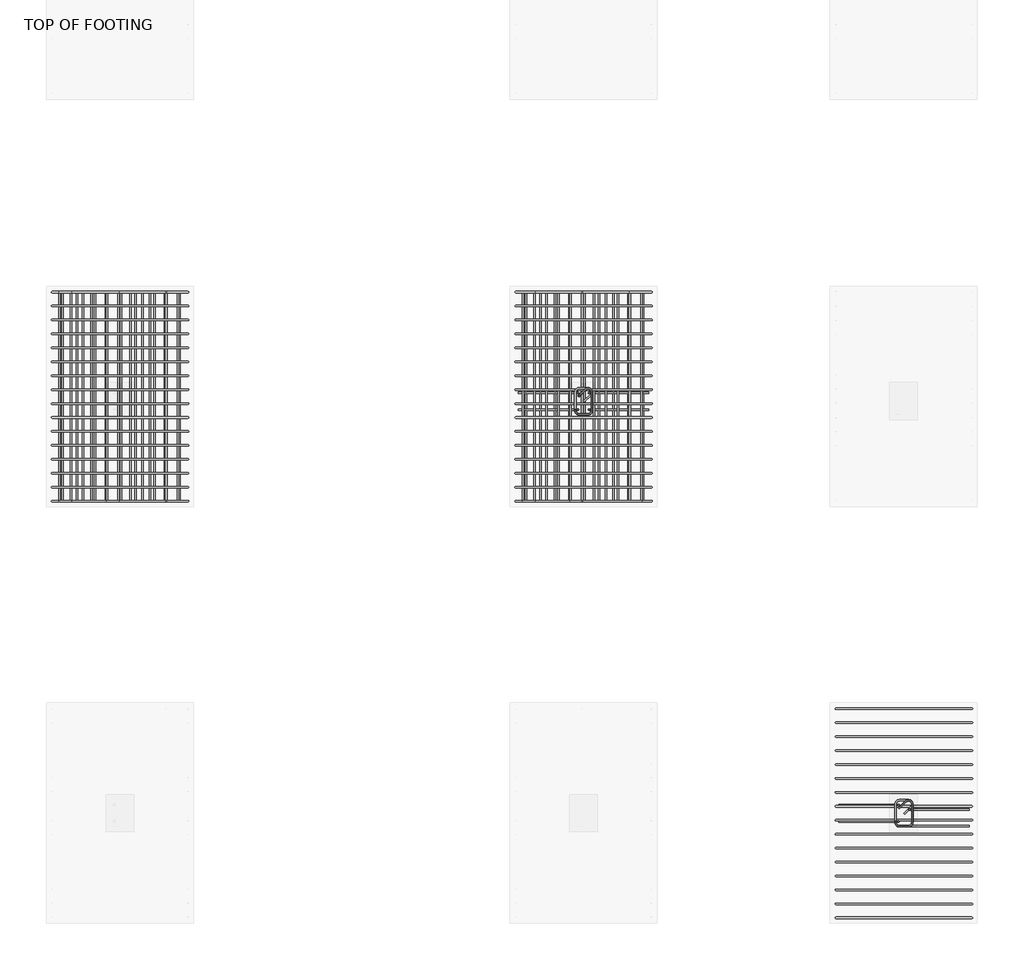
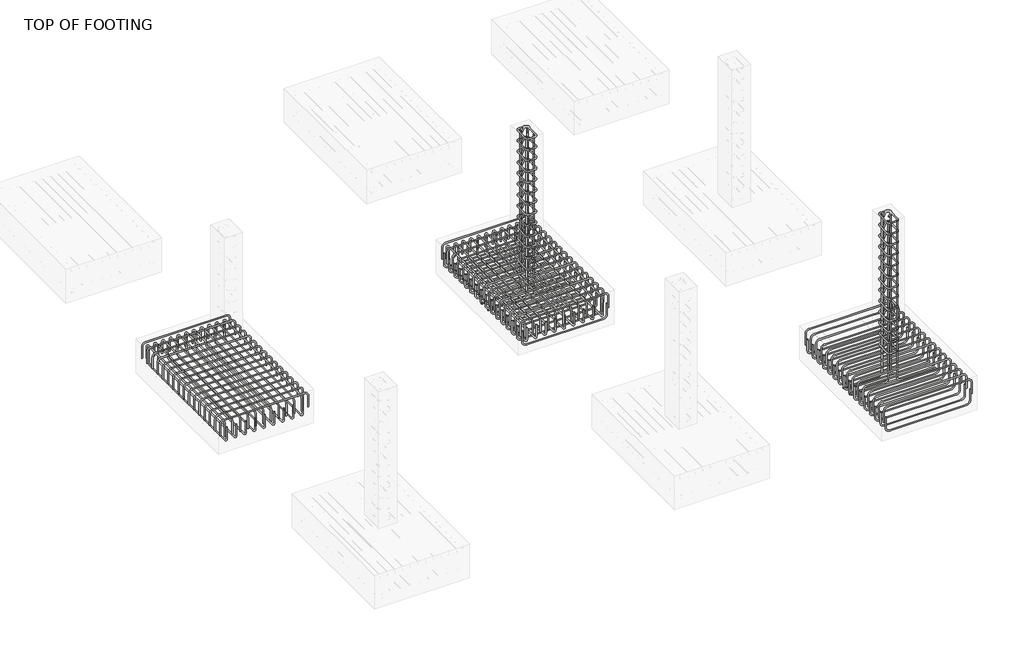
# One storey, part 6 of 8: 15 reinforcing bars.
"""IFC4 building model written with IfcOpenShell, lengths in millimetres."""

from ifc_helpers import new_model, si_unit, point, frame, origin, place, context, project, spatial, polyline, circle_curve, trimmed, segment, composite_curve, source, transform, mapped, element, save
from ifc_brep_helpers import swept_disk

model = new_model("IFC4")

# Units and contexts
model_context = context("Model", 3, world=origin())
ifc_project = project(units=[si_unit("LENGTHUNIT", "METRE", prefix="MILLI")], contexts=[model_context])

# Site, building, storey
site = spatial("IfcSite", under=ifc_project)
building = spatial("IfcBuilding", under=site)
storey = spatial("IfcBuildingStorey", under=building, Name="TOP OF FOOTING", Elevation=-1828.8)

# Reinforcing bars
placement = place(None, origin())
reinforcing_bar_shape = source(origin(), model_context, "Body", "SolidModel", [
    swept_disk(composite_curve([segment(polyline([(9462.2817577, 2235.4007933, -46.35), (9518.0253207, 2291.1443562, -46.35)]), True, "CONTINUOUS"), segment(trimmed(circle_curve(frame((9540.1931183, 2268.9765586, -46.35), z_axis=(0.0, 0.0, -1.0), x_axis=(-22.167797599999176, 22.167797600000085, 0.0)), 31.35), [point((9518.0253207, 2291.1443562, -46.35))], [point((9571.5431183, 2268.9765586, -46.35))], True, "CARTESIAN"), True, "CONTINUOUS"), segment(polyline([(9571.5431183, 2268.9765586, -46.35), (9571.5431183, 2119.5765586, -46.35)]), True, "CONTINUOUS"), segment(trimmed(circle_curve(frame((9540.1931183, 2119.5765586, -46.35), z_axis=(0.0, 0.0, -1.0), x_axis=(31.350000000000364, 0.0, 0.0)), 31.35), [point((9571.5431183, 2119.5765586, -46.35))], [point((9540.1931183, 2088.2265586, -46.35))], True, "CARTESIAN"), True, "CONTINUOUS"), segment(polyline([(9540.1931183, 2088.2265586, -46.35), (9466.9931183, 2088.2265586, -46.35)]), True, "CONTINUOUS"), segment(trimmed(circle_curve(frame((9466.9931183, 2119.5205096, -44.4761991), z_axis=(0.0, 0.05977036468717588, -0.9982121535551258), x_axis=(0.0, -31.293951000000106, -1.873800899999999)), 31.35), [point((9466.9931183, 2088.2265586, -46.35))], [point((9435.6431183, 2119.5205096, -44.4761991))], True, "CARTESIAN"), True, "CONTINUOUS"), segment(polyline([(9435.6431183, 2119.5205096, -44.4761991), (9435.6431183, 2269.0326076, -35.5238009)]), True, "CONTINUOUS"), segment(trimmed(circle_curve(frame((9466.9931183, 2269.0326076, -35.5238009), z_axis=(0.0, 0.05977036468717588, -0.9982121535551258), x_axis=(-31.350000000000364, 0.0, 0.0)), 31.35), [point((9435.6431183, 2269.0326076, -35.5238009))], [point((9466.9931183, 2300.3265586, -33.65))], True, "CARTESIAN"), True, "CONTINUOUS"), segment(polyline([(9466.9931183, 2300.3265586, -33.65), (9540.1931183, 2300.3265586, -33.65)]), True, "CONTINUOUS"), segment(trimmed(circle_curve(frame((9540.1931183, 2268.9765586, -33.65), z_axis=(0.0, 0.0, -1.0), x_axis=(0.0, 31.350000000000364, 0.0)), 31.35), [point((9540.1931183, 2300.3265586, -33.65))], [point((9562.3609159, 2246.808761, -33.65))], True, "CARTESIAN"), True, "CONTINUOUS"), segment(polyline([(9562.3609159, 2246.808761, -33.65), (9506.6173529, 2191.0651981, -33.65)]), True, "CONTINUOUS")], self_intersect=False), 6.35),
])
element("IfcReinforcingBar", 1, at=placement, inside=storey, context=model_context, shape_type="MappedRepresentation", body=[
    mapped(reinforcing_bar_shape, transform((0.0, 0.0, 0.0), x_axis=(1.0, 0.0, 0.0), y_axis=(0.0, 1.0, 0.0), z_axis=(0.0, 0.0, 1.0))),
    mapped(reinforcing_bar_shape, transform((0.0, 0.0, -144.675), x_axis=(1.0, 0.0, 0.0), y_axis=(0.0, 1.0, 0.0), z_axis=(0.0, 0.0, 1.0))),
    mapped(reinforcing_bar_shape, transform((0.0, 0.0, -289.35), x_axis=(1.0, 0.0, 0.0), y_axis=(0.0, 1.0, 0.0), z_axis=(0.0, 0.0, 1.0))),
    mapped(reinforcing_bar_shape, transform((0.0, 0.0, -434.025), x_axis=(1.0, 0.0, 0.0), y_axis=(0.0, 1.0, 0.0), z_axis=(0.0, 0.0, 1.0))),
    mapped(reinforcing_bar_shape, transform((0.0, 0.0, -578.7), x_axis=(1.0, 0.0, 0.0), y_axis=(0.0, 1.0, 0.0), z_axis=(0.0, 0.0, 1.0))),
    mapped(reinforcing_bar_shape, transform((0.0, 0.0, -723.375), x_axis=(1.0, 0.0, 0.0), y_axis=(0.0, 1.0, 0.0), z_axis=(0.0, 0.0, 1.0))),
    mapped(reinforcing_bar_shape, transform((0.0, 0.0, -868.05), x_axis=(1.0, 0.0, 0.0), y_axis=(0.0, 1.0, 0.0), z_axis=(0.0, 0.0, 1.0))),
    mapped(reinforcing_bar_shape, transform((0.0, 0.0, -1012.725), x_axis=(1.0, 0.0, 0.0), y_axis=(0.0, 1.0, 0.0), z_axis=(0.0, 0.0, 1.0))),
    mapped(reinforcing_bar_shape, transform((0.0, 0.0, -1157.4), x_axis=(1.0, 0.0, 0.0), y_axis=(0.0, 1.0, 0.0), z_axis=(0.0, 0.0, 1.0))),
    mapped(reinforcing_bar_shape, transform((0.0, 0.0, -1302.075), x_axis=(1.0, 0.0, 0.0), y_axis=(0.0, 1.0, 0.0), z_axis=(0.0, 0.0, 1.0))),
    mapped(reinforcing_bar_shape, transform((0.0, 0.0, -1446.75), x_axis=(1.0, 0.0, 0.0), y_axis=(0.0, 1.0, 0.0), z_axis=(0.0, 0.0, 1.0))),
    mapped(reinforcing_bar_shape, transform((0.0, 0.0, -1591.425), x_axis=(1.0, 0.0, 0.0), y_axis=(0.0, 1.0, 0.0), z_axis=(0.0, 0.0, 1.0))),
    mapped(reinforcing_bar_shape, transform((0.0, 0.0, -1736.1), x_axis=(1.0, 0.0, 0.0), y_axis=(0.0, 1.0, 0.0), z_axis=(0.0, 0.0, 1.0))),
])
reinforcing_bar_2_shape = source(origin(), model_context, "Body", "SolidModel", [
    swept_disk(composite_curve([segment(polyline([(10036.619602, 2088.2265586, -2177.1384798), (9595.4627797, 2088.2265586, -2177.1384798)]), True, "CONTINUOUS"), segment(trimmed(circle_curve(frame((9595.4627797, 2088.2265586, -2130.7884798), z_axis=(0.0, 1.0, 0.0), x_axis=(0.0, 0.0, -46.34999999999991)), 46.35), [point((9595.4627797, 2088.2265586, -2177.1384798))], [point((9549.1127797, 2088.2265586, -2130.7884798))], True, "CARTESIAN"), True, "CONTINUOUS"), segment(polyline([(9549.1127797, 2088.2265586, -2130.7884798), (9549.1127797, 2088.2265586, -40.0)]), True, "CONTINUOUS")], self_intersect=False), 6.35),
])
element("IfcReinforcingBar", 2, at=placement, inside=storey, context=model_context, shape_type="MappedRepresentation", body=[
    mapped(reinforcing_bar_2_shape, transform((0.0, 0.0, 0.0), x_axis=(1.0, 0.0, 0.0), y_axis=(0.0, 1.0, 0.0), z_axis=(0.0, 0.0, 1.0))),
    mapped(reinforcing_bar_2_shape, transform((0.0, 135.9, 0.0), x_axis=(1.0, 0.0, 0.0), y_axis=(0.0, 1.0, 0.0), z_axis=(0.0, 0.0, 1.0))),
])
reinforcing_bar_3_shape = source(origin(), model_context, "Body", "SolidModel", [
    swept_disk(composite_curve([segment(polyline([(8970.5666346, 2126.3265586, -2177.1384798), (9411.7234568, 2126.3265586, -2177.1384798)]), True, "CONTINUOUS"), segment(trimmed(circle_curve(frame((9411.7234568, 2126.3265586, -2130.7884798), z_axis=(0.0, -1.0, 0.0), x_axis=(0.0, 0.0, -46.34999999999991)), 46.35), [point((9411.7234568, 2126.3265586, -2177.1384798))], [point((9458.0734568, 2126.3265586, -2130.7884798))], True, "CARTESIAN"), True, "CONTINUOUS"), segment(polyline([(9458.0734568, 2126.3265586, -2130.7884798), (9458.0734568, 2126.3265586, -40.0)]), True, "CONTINUOUS")], self_intersect=False), 6.35),
])
element("IfcReinforcingBar", 3, at=placement, inside=storey, context=model_context, shape_type="MappedRepresentation", body=[
    mapped(reinforcing_bar_3_shape, transform((0.0, 0.0, 0.0), x_axis=(1.0, 0.0, 0.0), y_axis=(0.0, 1.0, 0.0), z_axis=(0.0, 0.0, 1.0))),
    mapped(reinforcing_bar_3_shape, transform((0.0, 135.9, 0.0), x_axis=(1.0, 0.0, 0.0), y_axis=(0.0, 1.0, 0.0), z_axis=(0.0, 0.0, 1.0))),
])
reinforcing_bar_4_shape = source(origin(), model_context, "Body", "SolidModel", [
    swept_disk(composite_curve([segment(polyline([(6846.0817577, 5600.7423139, -46.35), (6901.8253207, 5656.4858768, -46.35)]), True, "CONTINUOUS"), segment(trimmed(circle_curve(frame((6923.9931183, 5634.3180792, -46.35), z_axis=(0.0, 0.0, -1.0), x_axis=(-22.167797600000085, 22.167797600000085, 0.0)), 31.35), [point((6901.8253207, 5656.4858768, -46.35))], [point((6955.3431183, 5634.3180792, -46.35))], True, "CARTESIAN"), True, "CONTINUOUS"), segment(polyline([(6955.3431183, 5634.3180792, -46.35), (6955.3431183, 5484.9180792, -46.35)]), True, "CONTINUOUS"), segment(trimmed(circle_curve(frame((6923.9931183, 5484.9180792, -46.35), z_axis=(0.0, 0.0, -1.0), x_axis=(31.350000000000364, 0.0, 0.0)), 31.35), [point((6955.3431183, 5484.9180792, -46.35))], [point((6923.9931183, 5453.5680792, -46.35))], True, "CARTESIAN"), True, "CONTINUOUS"), segment(polyline([(6923.9931183, 5453.5680792, -46.35), (6850.7931183, 5453.5680792, -46.35)]), True, "CONTINUOUS"), segment(trimmed(circle_curve(frame((6850.7931183, 5484.8620303, -44.4761991), z_axis=(0.0, 0.05977036468717588, -0.9982121535551258), x_axis=(0.0, -31.293951099999504, -1.873800899999999)), 31.35), [point((6850.7931183, 5453.5680792, -46.35))], [point((6819.4431183, 5484.8620303, -44.4761991))], True, "CARTESIAN"), True, "CONTINUOUS"), segment(polyline([(6819.4431183, 5484.8620303, -44.4761991), (6819.4431183, 5634.3741282, -35.5238009)]), True, "CONTINUOUS"), segment(trimmed(circle_curve(frame((6850.7931183, 5634.3741282, -35.5238009), z_axis=(0.0, 0.05977036468717588, -0.9982121535551258), x_axis=(-31.350000000000364, 0.0, 0.0)), 31.35), [point((6819.4431183, 5634.3741282, -35.5238009))], [point((6850.7931183, 5665.6680792, -33.65))], True, "CARTESIAN"), True, "CONTINUOUS"), segment(polyline([(6850.7931183, 5665.6680792, -33.65), (6923.9931183, 5665.6680792, -33.65)]), True, "CONTINUOUS"), segment(trimmed(circle_curve(frame((6923.9931183, 5634.3180792, -33.65), z_axis=(0.0, 0.0, -1.0), x_axis=(0.0, 31.349999999999454, 0.0)), 31.35), [point((6923.9931183, 5665.6680792, -33.65))], [point((6946.1609159, 5612.1502816, -33.65))], True, "CARTESIAN"), True, "CONTINUOUS"), segment(polyline([(6946.1609159, 5612.1502816, -33.65), (6890.4173529, 5556.4067187, -33.65)]), True, "CONTINUOUS")], self_intersect=False), 6.35),
])
element("IfcReinforcingBar", 4, at=placement, inside=storey, context=model_context, shape_type="MappedRepresentation", body=[
    mapped(reinforcing_bar_4_shape, transform((0.0, 0.0, 0.0), x_axis=(1.0, 0.0, 0.0), y_axis=(0.0, 1.0, 0.0), z_axis=(0.0, 0.0, 1.0))),
    mapped(reinforcing_bar_4_shape, transform((0.0, 0.0, -144.675), x_axis=(1.0, 0.0, 0.0), y_axis=(0.0, 1.0, 0.0), z_axis=(0.0, 0.0, 1.0))),
    mapped(reinforcing_bar_4_shape, transform((0.0, 0.0, -289.35), x_axis=(1.0, 0.0, 0.0), y_axis=(0.0, 1.0, 0.0), z_axis=(0.0, 0.0, 1.0))),
    mapped(reinforcing_bar_4_shape, transform((0.0, 0.0, -434.025), x_axis=(1.0, 0.0, 0.0), y_axis=(0.0, 1.0, 0.0), z_axis=(0.0, 0.0, 1.0))),
    mapped(reinforcing_bar_4_shape, transform((0.0, 0.0, -578.7), x_axis=(1.0, 0.0, 0.0), y_axis=(0.0, 1.0, 0.0), z_axis=(0.0, 0.0, 1.0))),
    mapped(reinforcing_bar_4_shape, transform((0.0, 0.0, -723.375), x_axis=(1.0, 0.0, 0.0), y_axis=(0.0, 1.0, 0.0), z_axis=(0.0, 0.0, 1.0))),
    mapped(reinforcing_bar_4_shape, transform((0.0, 0.0, -868.05), x_axis=(1.0, 0.0, 0.0), y_axis=(0.0, 1.0, 0.0), z_axis=(0.0, 0.0, 1.0))),
    mapped(reinforcing_bar_4_shape, transform((0.0, 0.0, -1012.725), x_axis=(1.0, 0.0, 0.0), y_axis=(0.0, 1.0, 0.0), z_axis=(0.0, 0.0, 1.0))),
    mapped(reinforcing_bar_4_shape, transform((0.0, 0.0, -1157.4), x_axis=(1.0, 0.0, 0.0), y_axis=(0.0, 1.0, 0.0), z_axis=(0.0, 0.0, 1.0))),
    mapped(reinforcing_bar_4_shape, transform((0.0, 0.0, -1302.075), x_axis=(1.0, 0.0, 0.0), y_axis=(0.0, 1.0, 0.0), z_axis=(0.0, 0.0, 1.0))),
    mapped(reinforcing_bar_4_shape, transform((0.0, 0.0, -1446.75), x_axis=(1.0, 0.0, 0.0), y_axis=(0.0, 1.0, 0.0), z_axis=(0.0, 0.0, 1.0))),
    mapped(reinforcing_bar_4_shape, transform((0.0, 0.0, -1591.425), x_axis=(1.0, 0.0, 0.0), y_axis=(0.0, 1.0, 0.0), z_axis=(0.0, 0.0, 1.0))),
    mapped(reinforcing_bar_4_shape, transform((0.0, 0.0, -1736.1), x_axis=(1.0, 0.0, 0.0), y_axis=(0.0, 1.0, 0.0), z_axis=(0.0, 0.0, 1.0))),
])
reinforcing_bar_5_shape = source(origin(), model_context, "Body", "SolidModel", [
    swept_disk(composite_curve([segment(polyline([(7420.419602, 5491.6680792, -2177.1384798), (6979.2627797, 5491.6680792, -2177.1384798)]), True, "CONTINUOUS"), segment(trimmed(circle_curve(frame((6979.2627797, 5491.6680792, -2130.7884798), z_axis=(0.0, 1.0, 0.0), x_axis=(0.0, 0.0, -46.34999999999991)), 46.35), [point((6979.2627797, 5491.6680792, -2177.1384798))], [point((6932.9127797, 5491.6680792, -2130.7884798))], True, "CARTESIAN"), True, "CONTINUOUS"), segment(polyline([(6932.9127797, 5491.6680792, -2130.7884798), (6932.9127797, 5491.6680792, -40.0)]), True, "CONTINUOUS")], self_intersect=False), 6.35),
])
element("IfcReinforcingBar", 5, at=placement, inside=storey, context=model_context, shape_type="MappedRepresentation", body=[
    mapped(reinforcing_bar_5_shape, transform((0.0, 0.0, 0.0), x_axis=(1.0, 0.0, 0.0), y_axis=(0.0, 1.0, 0.0), z_axis=(0.0, 0.0, 1.0))),
    mapped(reinforcing_bar_5_shape, transform((0.0, 135.9, 0.0), x_axis=(1.0, 0.0, 0.0), y_axis=(0.0, 1.0, 0.0), z_axis=(0.0, 0.0, 1.0))),
])
reinforcing_bar_6_shape = source(origin(), model_context, "Body", "SolidModel", [
    swept_disk(composite_curve([segment(polyline([(6354.3666346, 5491.6680792, -2177.1384798), (6795.5234568, 5491.6680792, -2177.1384798)]), True, "CONTINUOUS"), segment(trimmed(circle_curve(frame((6795.5234568, 5491.6680792, -2130.7884798), z_axis=(0.0, -1.0, 0.0), x_axis=(0.0, 0.0, -46.34999999999991)), 46.35), [point((6795.5234568, 5491.6680792, -2177.1384798))], [point((6841.8734568, 5491.6680792, -2130.7884798))], True, "CARTESIAN"), True, "CONTINUOUS"), segment(polyline([(6841.8734568, 5491.6680792, -2130.7884798), (6841.8734568, 5491.6680792, -40.0)]), True, "CONTINUOUS")], self_intersect=False), 6.35),
])
element("IfcReinforcingBar", 6, at=placement, inside=storey, context=model_context, shape_type="MappedRepresentation", body=[
    mapped(reinforcing_bar_6_shape, transform((0.0, 0.0, 0.0), x_axis=(1.0, 0.0, 0.0), y_axis=(0.0, 1.0, 0.0), z_axis=(0.0, 0.0, 1.0))),
    mapped(reinforcing_bar_6_shape, transform((0.0, 135.9, 0.0), x_axis=(1.0, 0.0, 0.0), y_axis=(0.0, 1.0, 0.0), z_axis=(0.0, 0.0, 1.0))),
])
reinforcing_bar_7_shape = source(origin(), model_context, "Body", "SolidModel", [
    swept_disk(composite_curve([segment(polyline([(2549.1431183, 6451.7662126, -2068.8), (2549.1431183, 6451.7662126, -1921.5)]), True, "CONTINUOUS"), segment(trimmed(circle_curve(frame((2595.4931183, 6451.7662126, -1921.5), z_axis=(0.0, 1.0, 0.0), x_axis=(-46.34999999999991, 0.0, 0.0)), 46.35), [point((2549.1431183, 6451.7662126, -1921.5))], [point((2595.4931183, 6451.7662126, -1875.15))], True, "CARTESIAN"), True, "CONTINUOUS"), segment(polyline([(2595.4931183, 6451.7662126, -1875.15), (3610.0931183, 6451.7662126, -1875.15)]), True, "CONTINUOUS"), segment(trimmed(circle_curve(frame((3610.0931183, 6451.7662126, -1921.5), z_axis=(0.0, 1.0, 0.0), x_axis=(0.0, 0.0, 46.34999999999991)), 46.35), [point((3610.0931183, 6451.7662126, -1875.15))], [point((3656.4431183, 6451.7662126, -1921.5))], True, "CARTESIAN"), True, "CONTINUOUS"), segment(polyline([(3656.4431183, 6451.7662126, -1921.5), (3656.4431183, 6451.7662126, -2068.8)]), True, "CONTINUOUS")], self_intersect=False), 6.35),
])
element("IfcReinforcingBar", 7, at=placement, inside=storey, context=model_context, shape_type="MappedRepresentation", body=[
    mapped(reinforcing_bar_7_shape, transform((0.0, 0.0, 0.0), x_axis=(1.0, 0.0, 0.0), y_axis=(0.0, 1.0, 0.0), z_axis=(0.0, 0.0, 1.0))),
    mapped(reinforcing_bar_7_shape, transform((0.0, -113.82, 0.0), x_axis=(1.0, 0.0, 0.0), y_axis=(0.0, 1.0, 0.0), z_axis=(0.0, 0.0, 1.0))),
    mapped(reinforcing_bar_7_shape, transform((0.0, -227.64, 0.0), x_axis=(1.0, 0.0, 0.0), y_axis=(0.0, 1.0, 0.0), z_axis=(0.0, 0.0, 1.0))),
    mapped(reinforcing_bar_7_shape, transform((0.0, -341.46, 0.0), x_axis=(1.0, 0.0, 0.0), y_axis=(0.0, 1.0, 0.0), z_axis=(0.0, 0.0, 1.0))),
    mapped(reinforcing_bar_7_shape, transform((0.0, -455.28, 0.0), x_axis=(1.0, 0.0, 0.0), y_axis=(0.0, 1.0, 0.0), z_axis=(0.0, 0.0, 1.0))),
    mapped(reinforcing_bar_7_shape, transform((0.0, -569.1, 0.0), x_axis=(1.0, 0.0, 0.0), y_axis=(0.0, 1.0, 0.0), z_axis=(0.0, 0.0, 1.0))),
    mapped(reinforcing_bar_7_shape, transform((0.0, -682.92, 0.0), x_axis=(1.0, 0.0, 0.0), y_axis=(0.0, 1.0, 0.0), z_axis=(0.0, 0.0, 1.0))),
    mapped(reinforcing_bar_7_shape, transform((0.0, -796.74, 0.0), x_axis=(1.0, 0.0, 0.0), y_axis=(0.0, 1.0, 0.0), z_axis=(0.0, 0.0, 1.0))),
    mapped(reinforcing_bar_7_shape, transform((0.0, -910.56, 0.0), x_axis=(1.0, 0.0, 0.0), y_axis=(0.0, 1.0, 0.0), z_axis=(0.0, 0.0, 1.0))),
    mapped(reinforcing_bar_7_shape, transform((0.0, -1024.38, 0.0), x_axis=(1.0, 0.0, 0.0), y_axis=(0.0, 1.0, 0.0), z_axis=(0.0, 0.0, 1.0))),
    mapped(reinforcing_bar_7_shape, transform((0.0, -1138.2, 0.0), x_axis=(1.0, 0.0, 0.0), y_axis=(0.0, 1.0, 0.0), z_axis=(0.0, 0.0, 1.0))),
    mapped(reinforcing_bar_7_shape, transform((0.0, -1252.02, 0.0), x_axis=(1.0, 0.0, 0.0), y_axis=(0.0, 1.0, 0.0), z_axis=(0.0, 0.0, 1.0))),
    mapped(reinforcing_bar_7_shape, transform((0.0, -1365.84, 0.0), x_axis=(1.0, 0.0, 0.0), y_axis=(0.0, 1.0, 0.0), z_axis=(0.0, 0.0, 1.0))),
    mapped(reinforcing_bar_7_shape, transform((0.0, -1479.66, 0.0), x_axis=(1.0, 0.0, 0.0), y_axis=(0.0, 1.0, 0.0), z_axis=(0.0, 0.0, 1.0))),
    mapped(reinforcing_bar_7_shape, transform((0.0, -1593.48, 0.0), x_axis=(1.0, 0.0, 0.0), y_axis=(0.0, 1.0, 0.0), z_axis=(0.0, 0.0, 1.0))),
    mapped(reinforcing_bar_7_shape, transform((0.0, -1707.3, 0.0), x_axis=(1.0, 0.0, 0.0), y_axis=(0.0, 1.0, 0.0), z_axis=(0.0, 0.0, 1.0))),
])
reinforcing_bar_8_shape = source(origin(), model_context, "Body", "SolidModel", [
    swept_disk(composite_curve([segment(polyline([(2631.3651697, 6451.7662126, -1986.9111268), (2631.3651697, 6451.7662126, -2134.2111268)]), True, "CONTINUOUS"), segment(trimmed(circle_curve(frame((2631.3651697, 6405.4162126, -2134.2111268), z_axis=(-1.0, 0.0, 0.0), x_axis=(0.0, 46.349999999999454, 0.0)), 46.35), [point((2631.3651697, 6451.7662126, -2134.2111268))], [point((2631.3651697, 6405.4162126, -2180.5611268))], True, "CARTESIAN"), True, "CONTINUOUS"), segment(polyline([(2631.3651697, 6405.4162126, -2180.5611268), (2631.3651697, 4790.8162126, -2180.5611268)]), True, "CONTINUOUS"), segment(trimmed(circle_curve(frame((2631.3651697, 4790.8162126, -2134.2111268), z_axis=(-1.0, 0.0, 0.0), x_axis=(0.0, 0.0, -46.34999999999991)), 46.35), [point((2631.3651697, 4790.8162126, -2180.5611268))], [point((2631.3651697, 4744.4662126, -2134.2111268))], True, "CARTESIAN"), True, "CONTINUOUS"), segment(polyline([(2631.3651697, 4744.4662126, -2134.2111268), (2631.3651697, 4744.4662126, -1986.9111268)]), True, "CONTINUOUS")], self_intersect=False), 6.35),
])
element("IfcReinforcingBar", 8, at=placement, inside=storey, context=model_context, shape_type="MappedRepresentation", body=[
    mapped(reinforcing_bar_8_shape, transform((0.0, 0.0, 0.0), x_axis=(1.0, 0.0, 0.0), y_axis=(0.0, 1.0, 0.0), z_axis=(0.0, 0.0, 1.0))),
    mapped(reinforcing_bar_8_shape, transform((119.5564677, 0.0, 0.0), x_axis=(1.0, 0.0, 0.0), y_axis=(0.0, 1.0, 0.0), z_axis=(0.0, 0.0, 1.0))),
    mapped(reinforcing_bar_8_shape, transform((239.1129355, 0.0, 0.0), x_axis=(1.0, 0.0, 0.0), y_axis=(0.0, 1.0, 0.0), z_axis=(0.0, 0.0, 1.0))),
    mapped(reinforcing_bar_8_shape, transform((358.6694032, 0.0, 0.0), x_axis=(1.0, 0.0, 0.0), y_axis=(0.0, 1.0, 0.0), z_axis=(0.0, 0.0, 1.0))),
    mapped(reinforcing_bar_8_shape, transform((478.2258709, 0.0, 0.0), x_axis=(1.0, 0.0, 0.0), y_axis=(0.0, 1.0, 0.0), z_axis=(0.0, 0.0, 1.0))),
    mapped(reinforcing_bar_8_shape, transform((597.7823387, 0.0, 0.0), x_axis=(1.0, 0.0, 0.0), y_axis=(0.0, 1.0, 0.0), z_axis=(0.0, 0.0, 1.0))),
    mapped(reinforcing_bar_8_shape, transform((717.3388064, 0.0, 0.0), x_axis=(1.0, 0.0, 0.0), y_axis=(0.0, 1.0, 0.0), z_axis=(0.0, 0.0, 1.0))),
    mapped(reinforcing_bar_8_shape, transform((836.8952741, 0.0, 0.0), x_axis=(1.0, 0.0, 0.0), y_axis=(0.0, 1.0, 0.0), z_axis=(0.0, 0.0, 1.0))),
    mapped(reinforcing_bar_8_shape, transform((956.4517419, 0.0, 0.0), x_axis=(1.0, 0.0, 0.0), y_axis=(0.0, 1.0, 0.0), z_axis=(0.0, 0.0, 1.0))),
])
reinforcing_bar_9_shape = source(origin(), model_context, "Body", "SolidModel", [
    swept_disk(composite_curve([segment(polyline([(3577.1331701, 6451.7662126, -2094.8977257), (3577.1331701, 6451.7662126, -1947.5977257)]), True, "CONTINUOUS"), segment(trimmed(circle_curve(frame((3577.1331701, 6405.4162126, -1947.5977257), z_axis=(1.0, 0.0, 0.0), x_axis=(0.0, 46.349999999999454, 0.0)), 46.35), [point((3577.1331701, 6451.7662126, -1947.5977257))], [point((3577.1331701, 6405.4162126, -1901.2477257))], True, "CARTESIAN"), True, "CONTINUOUS"), segment(polyline([(3577.1331701, 6405.4162126, -1901.2477257), (3577.1331701, 4790.8162126, -1901.2477257)]), True, "CONTINUOUS"), segment(trimmed(circle_curve(frame((3577.1331701, 4790.8162126, -1947.5977257), z_axis=(1.0, 0.0, 0.0), x_axis=(0.0, 0.0, 46.34999999999991)), 46.35), [point((3577.1331701, 4790.8162126, -1901.2477257))], [point((3577.1331701, 4744.4662126, -1947.5977257))], True, "CARTESIAN"), True, "CONTINUOUS"), segment(polyline([(3577.1331701, 4744.4662126, -1947.5977257), (3577.1331701, 4744.4662126, -2094.8977257)]), True, "CONTINUOUS")], self_intersect=False), 6.35),
])
element("IfcReinforcingBar", 9, at=placement, inside=storey, context=model_context, shape_type="MappedRepresentation", body=[
    mapped(reinforcing_bar_9_shape, transform((0.0, 0.0, 0.0), x_axis=(1.0, 0.0, 0.0), y_axis=(0.0, 1.0, 0.0), z_axis=(0.0, 0.0, 1.0))),
    mapped(reinforcing_bar_9_shape, transform((-97.0050815, 0.0, 0.0), x_axis=(1.0, 0.0, 0.0), y_axis=(0.0, 1.0, 0.0), z_axis=(0.0, 0.0, 1.0))),
    mapped(reinforcing_bar_9_shape, transform((-194.0101631, 0.0, 0.0), x_axis=(1.0, 0.0, 0.0), y_axis=(0.0, 1.0, 0.0), z_axis=(0.0, 0.0, 1.0))),
    mapped(reinforcing_bar_9_shape, transform((-291.0152446, 0.0, 0.0), x_axis=(1.0, 0.0, 0.0), y_axis=(0.0, 1.0, 0.0), z_axis=(0.0, 0.0, 1.0))),
    mapped(reinforcing_bar_9_shape, transform((-388.0203261, 0.0, 0.0), x_axis=(1.0, 0.0, 0.0), y_axis=(0.0, 1.0, 0.0), z_axis=(0.0, 0.0, 1.0))),
    mapped(reinforcing_bar_9_shape, transform((-485.0254076, 0.0, 0.0), x_axis=(1.0, 0.0, 0.0), y_axis=(0.0, 1.0, 0.0), z_axis=(0.0, 0.0, 1.0))),
    mapped(reinforcing_bar_9_shape, transform((-582.0304892, 0.0, 0.0), x_axis=(1.0, 0.0, 0.0), y_axis=(0.0, 1.0, 0.0), z_axis=(0.0, 0.0, 1.0))),
    mapped(reinforcing_bar_9_shape, transform((-679.0355707, 0.0, 0.0), x_axis=(1.0, 0.0, 0.0), y_axis=(0.0, 1.0, 0.0), z_axis=(0.0, 0.0, 1.0))),
    mapped(reinforcing_bar_9_shape, transform((-776.0406522, 0.0, 0.0), x_axis=(1.0, 0.0, 0.0), y_axis=(0.0, 1.0, 0.0), z_axis=(0.0, 0.0, 1.0))),
    mapped(reinforcing_bar_9_shape, transform((-873.0457338, 0.0, 0.0), x_axis=(1.0, 0.0, 0.0), y_axis=(0.0, 1.0, 0.0), z_axis=(0.0, 0.0, 1.0))),
    mapped(reinforcing_bar_9_shape, transform((-970.0508153, 0.0, 0.0), x_axis=(1.0, 0.0, 0.0), y_axis=(0.0, 1.0, 0.0), z_axis=(0.0, 0.0, 1.0))),
])
reinforcing_bar_10_shape = source(origin(), model_context, "Body", "SolidModel", [
    swept_disk(composite_curve([segment(polyline([(7421.6426771, 6451.7662126, -2008.2544267), (7421.6426771, 6451.7662126, -2155.5544267)]), True, "CONTINUOUS"), segment(trimmed(circle_curve(frame((7375.2926771, 6451.7662126, -2155.5544267), z_axis=(0.0, 1.0, 0.0), x_axis=(46.349999999999454, 0.0, 0.0)), 46.35), [point((7421.6426771, 6451.7662126, -2155.5544267))], [point((7375.2926771, 6451.7662126, -2201.9044267))], True, "CARTESIAN"), True, "CONTINUOUS"), segment(polyline([(7375.2926771, 6451.7662126, -2201.9044267), (6404.2766408, 6451.7662126, -2201.9044267)]), True, "CONTINUOUS"), segment(trimmed(circle_curve(frame((6404.2766408, 6451.7662126, -2155.5544267), z_axis=(0.0, 1.0, 0.0), x_axis=(0.0, 0.0, -46.34999999999991)), 46.35), [point((6404.2766408, 6451.7662126, -2201.9044267))], [point((6357.9266408, 6451.7662126, -2155.5544267))], True, "CARTESIAN"), True, "CONTINUOUS"), segment(polyline([(6357.9266408, 6451.7662126, -2155.5544267), (6357.9266408, 6451.7662126, -2008.2544267)]), True, "CONTINUOUS")], self_intersect=False), 6.35),
])
element("IfcReinforcingBar", 10, at=placement, inside=storey, context=model_context, shape_type="MappedRepresentation", body=[
    mapped(reinforcing_bar_10_shape, transform((0.0, 0.0, 0.0), x_axis=(1.0, 0.0, 0.0), y_axis=(0.0, 1.0, 0.0), z_axis=(0.0, 0.0, 1.0))),
    mapped(reinforcing_bar_10_shape, transform((0.0, -113.82, 0.0), x_axis=(1.0, 0.0, 0.0), y_axis=(0.0, 1.0, 0.0), z_axis=(0.0, 0.0, 1.0))),
    mapped(reinforcing_bar_10_shape, transform((0.0, -227.64, 0.0), x_axis=(1.0, 0.0, 0.0), y_axis=(0.0, 1.0, 0.0), z_axis=(0.0, 0.0, 1.0))),
    mapped(reinforcing_bar_10_shape, transform((0.0, -341.46, 0.0), x_axis=(1.0, 0.0, 0.0), y_axis=(0.0, 1.0, 0.0), z_axis=(0.0, 0.0, 1.0))),
    mapped(reinforcing_bar_10_shape, transform((0.0, -455.28, 0.0), x_axis=(1.0, 0.0, 0.0), y_axis=(0.0, 1.0, 0.0), z_axis=(0.0, 0.0, 1.0))),
    mapped(reinforcing_bar_10_shape, transform((0.0, -569.1, 0.0), x_axis=(1.0, 0.0, 0.0), y_axis=(0.0, 1.0, 0.0), z_axis=(0.0, 0.0, 1.0))),
    mapped(reinforcing_bar_10_shape, transform((0.0, -682.92, 0.0), x_axis=(1.0, 0.0, 0.0), y_axis=(0.0, 1.0, 0.0), z_axis=(0.0, 0.0, 1.0))),
    mapped(reinforcing_bar_10_shape, transform((0.0, -796.74, 0.0), x_axis=(1.0, 0.0, 0.0), y_axis=(0.0, 1.0, 0.0), z_axis=(0.0, 0.0, 1.0))),
    mapped(reinforcing_bar_10_shape, transform((0.0, -910.56, 0.0), x_axis=(1.0, 0.0, 0.0), y_axis=(0.0, 1.0, 0.0), z_axis=(0.0, 0.0, 1.0))),
    mapped(reinforcing_bar_10_shape, transform((0.0, -1024.38, 0.0), x_axis=(1.0, 0.0, 0.0), y_axis=(0.0, 1.0, 0.0), z_axis=(0.0, 0.0, 1.0))),
    mapped(reinforcing_bar_10_shape, transform((0.0, -1138.2, 0.0), x_axis=(1.0, 0.0, 0.0), y_axis=(0.0, 1.0, 0.0), z_axis=(0.0, 0.0, 1.0))),
    mapped(reinforcing_bar_10_shape, transform((0.0, -1252.02, 0.0), x_axis=(1.0, 0.0, 0.0), y_axis=(0.0, 1.0, 0.0), z_axis=(0.0, 0.0, 1.0))),
    mapped(reinforcing_bar_10_shape, transform((0.0, -1365.84, 0.0), x_axis=(1.0, 0.0, 0.0), y_axis=(0.0, 1.0, 0.0), z_axis=(0.0, 0.0, 1.0))),
    mapped(reinforcing_bar_10_shape, transform((0.0, -1479.66, 0.0), x_axis=(1.0, 0.0, 0.0), y_axis=(0.0, 1.0, 0.0), z_axis=(0.0, 0.0, 1.0))),
    mapped(reinforcing_bar_10_shape, transform((0.0, -1593.48, 0.0), x_axis=(1.0, 0.0, 0.0), y_axis=(0.0, 1.0, 0.0), z_axis=(0.0, 0.0, 1.0))),
    mapped(reinforcing_bar_10_shape, transform((0.0, -1707.3, 0.0), x_axis=(1.0, 0.0, 0.0), y_axis=(0.0, 1.0, 0.0), z_axis=(0.0, 0.0, 1.0))),
])
reinforcing_bar_11_shape = source(origin(), model_context, "Body", "SolidModel", [
    swept_disk(composite_curve([segment(polyline([(6333.7431183, 6451.7662126, -2068.8), (6333.7431183, 6451.7662126, -1921.5)]), True, "CONTINUOUS"), segment(trimmed(circle_curve(frame((6380.0931183, 6451.7662126, -1921.5), z_axis=(0.0, 1.0, 0.0), x_axis=(-46.350000000000364, 0.0, 0.0)), 46.35), [point((6333.7431183, 6451.7662126, -1921.5))], [point((6380.0931183, 6451.7662126, -1875.15))], True, "CARTESIAN"), True, "CONTINUOUS"), segment(polyline([(6380.0931183, 6451.7662126, -1875.15), (7394.6931183, 6451.7662126, -1875.15)]), True, "CONTINUOUS"), segment(trimmed(circle_curve(frame((7394.6931183, 6451.7662126, -1921.5), z_axis=(0.0, 1.0, 0.0), x_axis=(0.0, 0.0, 46.34999999999991)), 46.35), [point((7394.6931183, 6451.7662126, -1875.15))], [point((7441.0431183, 6451.7662126, -1921.5))], True, "CARTESIAN"), True, "CONTINUOUS"), segment(polyline([(7441.0431183, 6451.7662126, -1921.5), (7441.0431183, 6451.7662126, -2068.8)]), True, "CONTINUOUS")], self_intersect=False), 6.35),
])
element("IfcReinforcingBar", 11, at=placement, inside=storey, context=model_context, shape_type="MappedRepresentation", body=[
    mapped(reinforcing_bar_11_shape, transform((0.0, 0.0, 0.0), x_axis=(1.0, 0.0, 0.0), y_axis=(0.0, 1.0, 0.0), z_axis=(0.0, 0.0, 1.0))),
    mapped(reinforcing_bar_11_shape, transform((0.0, -113.82, 0.0), x_axis=(1.0, 0.0, 0.0), y_axis=(0.0, 1.0, 0.0), z_axis=(0.0, 0.0, 1.0))),
    mapped(reinforcing_bar_11_shape, transform((0.0, -227.64, 0.0), x_axis=(1.0, 0.0, 0.0), y_axis=(0.0, 1.0, 0.0), z_axis=(0.0, 0.0, 1.0))),
    mapped(reinforcing_bar_11_shape, transform((0.0, -341.46, 0.0), x_axis=(1.0, 0.0, 0.0), y_axis=(0.0, 1.0, 0.0), z_axis=(0.0, 0.0, 1.0))),
    mapped(reinforcing_bar_11_shape, transform((0.0, -455.28, 0.0), x_axis=(1.0, 0.0, 0.0), y_axis=(0.0, 1.0, 0.0), z_axis=(0.0, 0.0, 1.0))),
    mapped(reinforcing_bar_11_shape, transform((0.0, -569.1, 0.0), x_axis=(1.0, 0.0, 0.0), y_axis=(0.0, 1.0, 0.0), z_axis=(0.0, 0.0, 1.0))),
    mapped(reinforcing_bar_11_shape, transform((0.0, -682.92, 0.0), x_axis=(1.0, 0.0, 0.0), y_axis=(0.0, 1.0, 0.0), z_axis=(0.0, 0.0, 1.0))),
    mapped(reinforcing_bar_11_shape, transform((0.0, -796.74, 0.0), x_axis=(1.0, 0.0, 0.0), y_axis=(0.0, 1.0, 0.0), z_axis=(0.0, 0.0, 1.0))),
    mapped(reinforcing_bar_11_shape, transform((0.0, -910.56, 0.0), x_axis=(1.0, 0.0, 0.0), y_axis=(0.0, 1.0, 0.0), z_axis=(0.0, 0.0, 1.0))),
    mapped(reinforcing_bar_11_shape, transform((0.0, -1024.38, 0.0), x_axis=(1.0, 0.0, 0.0), y_axis=(0.0, 1.0, 0.0), z_axis=(0.0, 0.0, 1.0))),
    mapped(reinforcing_bar_11_shape, transform((0.0, -1138.2, 0.0), x_axis=(1.0, 0.0, 0.0), y_axis=(0.0, 1.0, 0.0), z_axis=(0.0, 0.0, 1.0))),
    mapped(reinforcing_bar_11_shape, transform((0.0, -1252.02, 0.0), x_axis=(1.0, 0.0, 0.0), y_axis=(0.0, 1.0, 0.0), z_axis=(0.0, 0.0, 1.0))),
    mapped(reinforcing_bar_11_shape, transform((0.0, -1365.84, 0.0), x_axis=(1.0, 0.0, 0.0), y_axis=(0.0, 1.0, 0.0), z_axis=(0.0, 0.0, 1.0))),
    mapped(reinforcing_bar_11_shape, transform((0.0, -1479.66, 0.0), x_axis=(1.0, 0.0, 0.0), y_axis=(0.0, 1.0, 0.0), z_axis=(0.0, 0.0, 1.0))),
    mapped(reinforcing_bar_11_shape, transform((0.0, -1593.48, 0.0), x_axis=(1.0, 0.0, 0.0), y_axis=(0.0, 1.0, 0.0), z_axis=(0.0, 0.0, 1.0))),
    mapped(reinforcing_bar_11_shape, transform((0.0, -1707.3, 0.0), x_axis=(1.0, 0.0, 0.0), y_axis=(0.0, 1.0, 0.0), z_axis=(0.0, 0.0, 1.0))),
])
reinforcing_bar_12_shape = source(origin(), model_context, "Body", "SolidModel", [
    swept_disk(composite_curve([segment(polyline([(6415.9651697, 6451.7662126, -1986.9111268), (6415.9651697, 6451.7662126, -2134.2111268)]), True, "CONTINUOUS"), segment(trimmed(circle_curve(frame((6415.9651697, 6405.4162126, -2134.2111268), z_axis=(-1.0, 0.0, 0.0), x_axis=(0.0, 46.349999999999454, 0.0)), 46.35), [point((6415.9651697, 6451.7662126, -2134.2111268))], [point((6415.9651697, 6405.4162126, -2180.5611268))], True, "CARTESIAN"), True, "CONTINUOUS"), segment(polyline([(6415.9651697, 6405.4162126, -2180.5611268), (6415.9651697, 4790.8162126, -2180.5611268)]), True, "CONTINUOUS"), segment(trimmed(circle_curve(frame((6415.9651697, 4790.8162126, -2134.2111268), z_axis=(-1.0, 0.0, 0.0), x_axis=(0.0, 0.0, -46.34999999999991)), 46.35), [point((6415.9651697, 4790.8162126, -2180.5611268))], [point((6415.9651697, 4744.4662126, -2134.2111268))], True, "CARTESIAN"), True, "CONTINUOUS"), segment(polyline([(6415.9651697, 4744.4662126, -2134.2111268), (6415.9651697, 4744.4662126, -1986.9111268)]), True, "CONTINUOUS")], self_intersect=False), 6.35),
])
element("IfcReinforcingBar", 12, at=placement, inside=storey, context=model_context, shape_type="MappedRepresentation", body=[
    mapped(reinforcing_bar_12_shape, transform((0.0, 0.0, 0.0), x_axis=(1.0, 0.0, 0.0), y_axis=(0.0, 1.0, 0.0), z_axis=(0.0, 0.0, 1.0))),
    mapped(reinforcing_bar_12_shape, transform((119.5564677, 0.0, 0.0), x_axis=(1.0, 0.0, 0.0), y_axis=(0.0, 1.0, 0.0), z_axis=(0.0, 0.0, 1.0))),
    mapped(reinforcing_bar_12_shape, transform((239.1129355, 0.0, 0.0), x_axis=(1.0, 0.0, 0.0), y_axis=(0.0, 1.0, 0.0), z_axis=(0.0, 0.0, 1.0))),
    mapped(reinforcing_bar_12_shape, transform((358.6694032, 0.0, 0.0), x_axis=(1.0, 0.0, 0.0), y_axis=(0.0, 1.0, 0.0), z_axis=(0.0, 0.0, 1.0))),
    mapped(reinforcing_bar_12_shape, transform((478.2258709, 0.0, 0.0), x_axis=(1.0, 0.0, 0.0), y_axis=(0.0, 1.0, 0.0), z_axis=(0.0, 0.0, 1.0))),
    mapped(reinforcing_bar_12_shape, transform((597.7823387, 0.0, 0.0), x_axis=(1.0, 0.0, 0.0), y_axis=(0.0, 1.0, 0.0), z_axis=(0.0, 0.0, 1.0))),
    mapped(reinforcing_bar_12_shape, transform((717.3388064, 0.0, 0.0), x_axis=(1.0, 0.0, 0.0), y_axis=(0.0, 1.0, 0.0), z_axis=(0.0, 0.0, 1.0))),
    mapped(reinforcing_bar_12_shape, transform((836.8952741, 0.0, 0.0), x_axis=(1.0, 0.0, 0.0), y_axis=(0.0, 1.0, 0.0), z_axis=(0.0, 0.0, 1.0))),
    mapped(reinforcing_bar_12_shape, transform((956.4517419, 0.0, 0.0), x_axis=(1.0, 0.0, 0.0), y_axis=(0.0, 1.0, 0.0), z_axis=(0.0, 0.0, 1.0))),
])
reinforcing_bar_13_shape = source(origin(), model_context, "Body", "SolidModel", [
    swept_disk(composite_curve([segment(polyline([(7361.7331701, 6451.7662126, -2094.8977257), (7361.7331701, 6451.7662126, -1947.5977257)]), True, "CONTINUOUS"), segment(trimmed(circle_curve(frame((7361.7331701, 6405.4162126, -1947.5977257), z_axis=(1.0, 0.0, 0.0), x_axis=(0.0, 46.349999999999454, 0.0)), 46.35), [point((7361.7331701, 6451.7662126, -1947.5977257))], [point((7361.7331701, 6405.4162126, -1901.2477257))], True, "CARTESIAN"), True, "CONTINUOUS"), segment(polyline([(7361.7331701, 6405.4162126, -1901.2477257), (7361.7331701, 4790.8162126, -1901.2477257)]), True, "CONTINUOUS"), segment(trimmed(circle_curve(frame((7361.7331701, 4790.8162126, -1947.5977257), z_axis=(1.0, 0.0, 0.0), x_axis=(0.0, 0.0, 46.34999999999991)), 46.35), [point((7361.7331701, 4790.8162126, -1901.2477257))], [point((7361.7331701, 4744.4662126, -1947.5977257))], True, "CARTESIAN"), True, "CONTINUOUS"), segment(polyline([(7361.7331701, 4744.4662126, -1947.5977257), (7361.7331701, 4744.4662126, -2094.8977257)]), True, "CONTINUOUS")], self_intersect=False), 6.35),
])
element("IfcReinforcingBar", 13, at=placement, inside=storey, context=model_context, shape_type="MappedRepresentation", body=[
    mapped(reinforcing_bar_13_shape, transform((0.0, 0.0, 0.0), x_axis=(1.0, 0.0, 0.0), y_axis=(0.0, 1.0, 0.0), z_axis=(0.0, 0.0, 1.0))),
    mapped(reinforcing_bar_13_shape, transform((-97.0050815, 0.0, 0.0), x_axis=(1.0, 0.0, 0.0), y_axis=(0.0, 1.0, 0.0), z_axis=(0.0, 0.0, 1.0))),
    mapped(reinforcing_bar_13_shape, transform((-194.0101631, 0.0, 0.0), x_axis=(1.0, 0.0, 0.0), y_axis=(0.0, 1.0, 0.0), z_axis=(0.0, 0.0, 1.0))),
    mapped(reinforcing_bar_13_shape, transform((-291.0152446, 0.0, 0.0), x_axis=(1.0, 0.0, 0.0), y_axis=(0.0, 1.0, 0.0), z_axis=(0.0, 0.0, 1.0))),
    mapped(reinforcing_bar_13_shape, transform((-388.0203261, 0.0, 0.0), x_axis=(1.0, 0.0, 0.0), y_axis=(0.0, 1.0, 0.0), z_axis=(0.0, 0.0, 1.0))),
    mapped(reinforcing_bar_13_shape, transform((-485.0254076, 0.0, 0.0), x_axis=(1.0, 0.0, 0.0), y_axis=(0.0, 1.0, 0.0), z_axis=(0.0, 0.0, 1.0))),
    mapped(reinforcing_bar_13_shape, transform((-582.0304892, 0.0, 0.0), x_axis=(1.0, 0.0, 0.0), y_axis=(0.0, 1.0, 0.0), z_axis=(0.0, 0.0, 1.0))),
    mapped(reinforcing_bar_13_shape, transform((-679.0355707, 0.0, 0.0), x_axis=(1.0, 0.0, 0.0), y_axis=(0.0, 1.0, 0.0), z_axis=(0.0, 0.0, 1.0))),
    mapped(reinforcing_bar_13_shape, transform((-776.0406522, 0.0, 0.0), x_axis=(1.0, 0.0, 0.0), y_axis=(0.0, 1.0, 0.0), z_axis=(0.0, 0.0, 1.0))),
    mapped(reinforcing_bar_13_shape, transform((-873.0457338, 0.0, 0.0), x_axis=(1.0, 0.0, 0.0), y_axis=(0.0, 1.0, 0.0), z_axis=(0.0, 0.0, 1.0))),
    mapped(reinforcing_bar_13_shape, transform((-970.0508153, 0.0, 0.0), x_axis=(1.0, 0.0, 0.0), y_axis=(0.0, 1.0, 0.0), z_axis=(0.0, 0.0, 1.0))),
])
reinforcing_bar_14_shape = source(origin(), model_context, "Body", "SolidModel", [
    swept_disk(composite_curve([segment(polyline([(10037.8426771, 3047.9265586, -2008.2544267), (10037.8426771, 3047.9265586, -2155.5544267)]), True, "CONTINUOUS"), segment(trimmed(circle_curve(frame((9991.4926771, 3047.9265586, -2155.5544267), z_axis=(0.0, 1.0, 0.0), x_axis=(46.350000000000364, 0.0, 0.0)), 46.35), [point((10037.8426771, 3047.9265586, -2155.5544267))], [point((9991.4926771, 3047.9265586, -2201.9044267))], True, "CARTESIAN"), True, "CONTINUOUS"), segment(polyline([(9991.4926771, 3047.9265586, -2201.9044267), (9020.4766408, 3047.9265586, -2201.9044267)]), True, "CONTINUOUS"), segment(trimmed(circle_curve(frame((9020.4766408, 3047.9265586, -2155.5544267), z_axis=(0.0, 1.0, 0.0), x_axis=(0.0, 0.0, -46.34999999999991)), 46.35), [point((9020.4766408, 3047.9265586, -2201.9044267))], [point((8974.1266408, 3047.9265586, -2155.5544267))], True, "CARTESIAN"), True, "CONTINUOUS"), segment(polyline([(8974.1266408, 3047.9265586, -2155.5544267), (8974.1266408, 3047.9265586, -2008.2544267)]), True, "CONTINUOUS")], self_intersect=False), 6.35),
])
element("IfcReinforcingBar", 14, at=placement, inside=storey, context=model_context, shape_type="MappedRepresentation", body=[
    mapped(reinforcing_bar_14_shape, transform((0.0, 0.0, 0.0), x_axis=(1.0, 0.0, 0.0), y_axis=(0.0, 1.0, 0.0), z_axis=(0.0, 0.0, 1.0))),
    mapped(reinforcing_bar_14_shape, transform((0.0, -113.82, 0.0), x_axis=(1.0, 0.0, 0.0), y_axis=(0.0, 1.0, 0.0), z_axis=(0.0, 0.0, 1.0))),
    mapped(reinforcing_bar_14_shape, transform((0.0, -227.64, 0.0), x_axis=(1.0, 0.0, 0.0), y_axis=(0.0, 1.0, 0.0), z_axis=(0.0, 0.0, 1.0))),
    mapped(reinforcing_bar_14_shape, transform((0.0, -341.46, 0.0), x_axis=(1.0, 0.0, 0.0), y_axis=(0.0, 1.0, 0.0), z_axis=(0.0, 0.0, 1.0))),
    mapped(reinforcing_bar_14_shape, transform((0.0, -455.28, 0.0), x_axis=(1.0, 0.0, 0.0), y_axis=(0.0, 1.0, 0.0), z_axis=(0.0, 0.0, 1.0))),
    mapped(reinforcing_bar_14_shape, transform((0.0, -569.1, 0.0), x_axis=(1.0, 0.0, 0.0), y_axis=(0.0, 1.0, 0.0), z_axis=(0.0, 0.0, 1.0))),
    mapped(reinforcing_bar_14_shape, transform((0.0, -682.92, 0.0), x_axis=(1.0, 0.0, 0.0), y_axis=(0.0, 1.0, 0.0), z_axis=(0.0, 0.0, 1.0))),
    mapped(reinforcing_bar_14_shape, transform((0.0, -796.74, 0.0), x_axis=(1.0, 0.0, 0.0), y_axis=(0.0, 1.0, 0.0), z_axis=(0.0, 0.0, 1.0))),
    mapped(reinforcing_bar_14_shape, transform((0.0, -910.56, 0.0), x_axis=(1.0, 0.0, 0.0), y_axis=(0.0, 1.0, 0.0), z_axis=(0.0, 0.0, 1.0))),
    mapped(reinforcing_bar_14_shape, transform((0.0, -1024.38, 0.0), x_axis=(1.0, 0.0, 0.0), y_axis=(0.0, 1.0, 0.0), z_axis=(0.0, 0.0, 1.0))),
    mapped(reinforcing_bar_14_shape, transform((0.0, -1138.2, 0.0), x_axis=(1.0, 0.0, 0.0), y_axis=(0.0, 1.0, 0.0), z_axis=(0.0, 0.0, 1.0))),
    mapped(reinforcing_bar_14_shape, transform((0.0, -1252.02, 0.0), x_axis=(1.0, 0.0, 0.0), y_axis=(0.0, 1.0, 0.0), z_axis=(0.0, 0.0, 1.0))),
    mapped(reinforcing_bar_14_shape, transform((0.0, -1365.84, 0.0), x_axis=(1.0, 0.0, 0.0), y_axis=(0.0, 1.0, 0.0), z_axis=(0.0, 0.0, 1.0))),
    mapped(reinforcing_bar_14_shape, transform((0.0, -1479.66, 0.0), x_axis=(1.0, 0.0, 0.0), y_axis=(0.0, 1.0, 0.0), z_axis=(0.0, 0.0, 1.0))),
    mapped(reinforcing_bar_14_shape, transform((0.0, -1593.48, 0.0), x_axis=(1.0, 0.0, 0.0), y_axis=(0.0, 1.0, 0.0), z_axis=(0.0, 0.0, 1.0))),
    mapped(reinforcing_bar_14_shape, transform((0.0, -1707.3, 0.0), x_axis=(1.0, 0.0, 0.0), y_axis=(0.0, 1.0, 0.0), z_axis=(0.0, 0.0, 1.0))),
])
reinforcing_bar_15_shape = source(origin(), model_context, "Body", "SolidModel", [
    swept_disk(composite_curve([segment(polyline([(8949.9431183, 3047.9265586, -2068.8), (8949.9431183, 3047.9265586, -1921.5)]), True, "CONTINUOUS"), segment(trimmed(circle_curve(frame((8996.2931183, 3047.9265586, -1921.5), z_axis=(0.0, 1.0, 0.0), x_axis=(-46.350000000000364, 0.0, 0.0)), 46.35), [point((8949.9431183, 3047.9265586, -1921.5))], [point((8996.2931183, 3047.9265586, -1875.15))], True, "CARTESIAN"), True, "CONTINUOUS"), segment(polyline([(8996.2931183, 3047.9265586, -1875.15), (10010.8931183, 3047.9265586, -1875.15)]), True, "CONTINUOUS"), segment(trimmed(circle_curve(frame((10010.8931183, 3047.9265586, -1921.5), z_axis=(0.0, 1.0, 0.0), x_axis=(0.0, 0.0, 46.34999999999991)), 46.35), [point((10010.8931183, 3047.9265586, -1875.15))], [point((10057.2431183, 3047.9265586, -1921.5))], True, "CARTESIAN"), True, "CONTINUOUS"), segment(polyline([(10057.2431183, 3047.9265586, -1921.5), (10057.2431183, 3047.9265586, -2068.8)]), True, "CONTINUOUS")], self_intersect=False), 6.35),
])
element("IfcReinforcingBar", 15, at=placement, inside=storey, context=model_context, shape_type="MappedRepresentation", body=[
    mapped(reinforcing_bar_15_shape, transform((0.0, 0.0, 0.0), x_axis=(1.0, 0.0, 0.0), y_axis=(0.0, 1.0, 0.0), z_axis=(0.0, 0.0, 1.0))),
    mapped(reinforcing_bar_15_shape, transform((0.0, -113.82, 0.0), x_axis=(1.0, 0.0, 0.0), y_axis=(0.0, 1.0, 0.0), z_axis=(0.0, 0.0, 1.0))),
    mapped(reinforcing_bar_15_shape, transform((0.0, -227.64, 0.0), x_axis=(1.0, 0.0, 0.0), y_axis=(0.0, 1.0, 0.0), z_axis=(0.0, 0.0, 1.0))),
    mapped(reinforcing_bar_15_shape, transform((0.0, -341.46, 0.0), x_axis=(1.0, 0.0, 0.0), y_axis=(0.0, 1.0, 0.0), z_axis=(0.0, 0.0, 1.0))),
    mapped(reinforcing_bar_15_shape, transform((0.0, -455.28, 0.0), x_axis=(1.0, 0.0, 0.0), y_axis=(0.0, 1.0, 0.0), z_axis=(0.0, 0.0, 1.0))),
    mapped(reinforcing_bar_15_shape, transform((0.0, -569.1, 0.0), x_axis=(1.0, 0.0, 0.0), y_axis=(0.0, 1.0, 0.0), z_axis=(0.0, 0.0, 1.0))),
    mapped(reinforcing_bar_15_shape, transform((0.0, -682.92, 0.0), x_axis=(1.0, 0.0, 0.0), y_axis=(0.0, 1.0, 0.0), z_axis=(0.0, 0.0, 1.0))),
    mapped(reinforcing_bar_15_shape, transform((0.0, -796.74, 0.0), x_axis=(1.0, 0.0, 0.0), y_axis=(0.0, 1.0, 0.0), z_axis=(0.0, 0.0, 1.0))),
    mapped(reinforcing_bar_15_shape, transform((0.0, -910.56, 0.0), x_axis=(1.0, 0.0, 0.0), y_axis=(0.0, 1.0, 0.0), z_axis=(0.0, 0.0, 1.0))),
    mapped(reinforcing_bar_15_shape, transform((0.0, -1024.38, 0.0), x_axis=(1.0, 0.0, 0.0), y_axis=(0.0, 1.0, 0.0), z_axis=(0.0, 0.0, 1.0))),
    mapped(reinforcing_bar_15_shape, transform((0.0, -1138.2, 0.0), x_axis=(1.0, 0.0, 0.0), y_axis=(0.0, 1.0, 0.0), z_axis=(0.0, 0.0, 1.0))),
    mapped(reinforcing_bar_15_shape, transform((0.0, -1252.02, 0.0), x_axis=(1.0, 0.0, 0.0), y_axis=(0.0, 1.0, 0.0), z_axis=(0.0, 0.0, 1.0))),
    mapped(reinforcing_bar_15_shape, transform((0.0, -1365.84, 0.0), x_axis=(1.0, 0.0, 0.0), y_axis=(0.0, 1.0, 0.0), z_axis=(0.0, 0.0, 1.0))),
    mapped(reinforcing_bar_15_shape, transform((0.0, -1479.66, 0.0), x_axis=(1.0, 0.0, 0.0), y_axis=(0.0, 1.0, 0.0), z_axis=(0.0, 0.0, 1.0))),
    mapped(reinforcing_bar_15_shape, transform((0.0, -1593.48, 0.0), x_axis=(1.0, 0.0, 0.0), y_axis=(0.0, 1.0, 0.0), z_axis=(0.0, 0.0, 1.0))),
    mapped(reinforcing_bar_15_shape, transform((0.0, -1707.3, 0.0), x_axis=(1.0, 0.0, 0.0), y_axis=(0.0, 1.0, 0.0), z_axis=(0.0, 0.0, 1.0))),
])

save(model, "model.ifc")

# Revit data of these elements
# Elements 1, 2, 3, 4, 5, 6, 7, 8, 9, 10, 11, 12, 13, 14, 15 (IfcReinforcingBar)
#   Phase Created = New Construction
